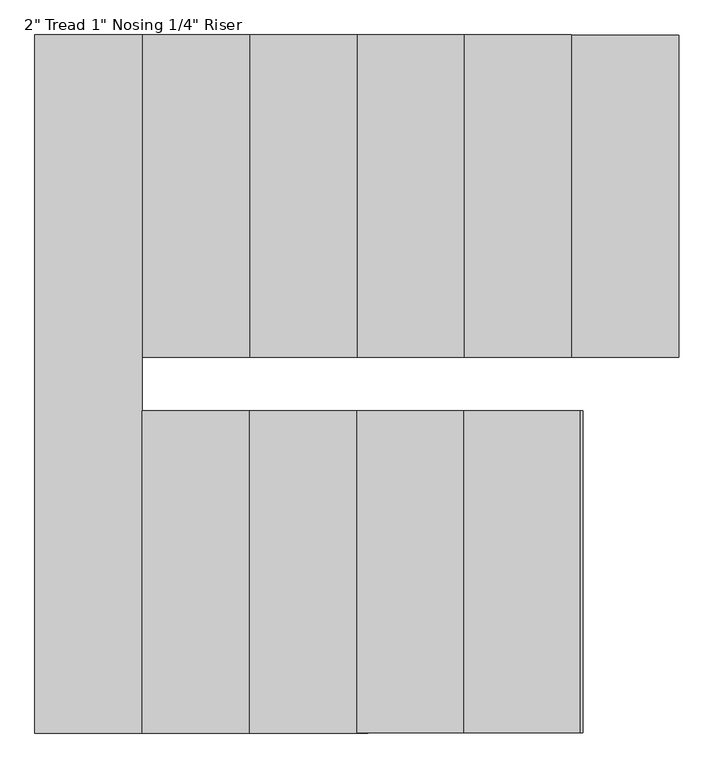
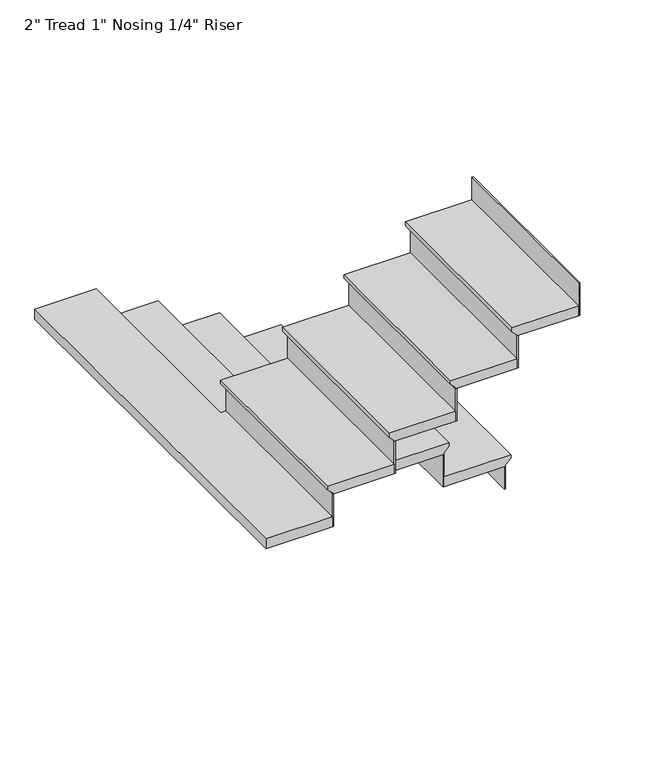
"""IFC4 building model written with IfcOpenShell, lengths in millimetres: stair flight geometry."""

from ifc_helpers import new_model, si_unit, origin, place, context, project, spatial, faceted_brep, source, transform, mapped, element, save


def stair_flight_2df44192(model_context):
    return source(origin(), model_context, "Body", "Brep", [
        faceted_brep([(3327.4, 3340.1, 6246.2833333), (3327.4, 3340.1, 6265.3333333), (3327.4, 2425.7, 6265.3333333), (3327.4, 2425.7, 6246.2833333), (3302.0, 3340.1, 6220.8833333), (3302.0, 2425.7, 6220.8833333), (2997.2, 3340.1, 6265.3333333), (2997.2, 2425.7, 6265.3333333), (3302.0, 2425.7, 6214.5333333), (2997.2, 2425.7, 6214.5333333), (2997.2, 3340.1, 6214.5333333), (3302.0, 3340.1, 6214.5333333)], [[[0, 1, 2, 3]], [[4, 0, 3, 5]], [[2, 1, 6, 7]], [[8, 9, 10, 11]], [[2, 7, 9, 8, 5, 3]], [[8, 11, 4, 5]], [[6, 1, 0, 4, 11, 10]], [[7, 6, 10, 9]]]),
        faceted_brep([(3302.0, 3340.1, 6214.5333333), (3302.0, 3340.1, 6096.0), (3295.65, 3340.1, 6096.0), (3295.65, 3340.1, 6214.5333333), (3302.0, 2425.7, 6214.5333333), (3295.65, 2425.7, 6214.5333333), (3295.65, 2425.7, 6096.0), (3302.0, 2425.7, 6096.0)], [[[0, 1, 2, 3]], [[4, 5, 6, 7]], [[1, 0, 4, 7]], [[2, 1, 7, 6]], [[3, 2, 6, 5]], [[0, 3, 5, 4]]]),
        faceted_brep([(2997.2, 3340.1, 6383.8666667), (2997.2, 3340.1, 6214.5333333), (2990.85, 3340.1, 6214.5333333), (2990.85, 3340.1, 6383.8666667), (2997.2, 2425.7, 6383.8666667), (2990.85, 2425.7, 6383.8666667), (2990.85, 2425.7, 6214.5333333), (2997.2, 2425.7, 6214.5333333)], [[[0, 1, 2, 3]], [[4, 5, 6, 7]], [[1, 0, 4, 7]], [[2, 1, 7, 6]], [[3, 2, 6, 5]], [[0, 3, 5, 4]]]),
        faceted_brep([(3022.6, 2425.7, 6434.6666667), (3022.6, 3340.1, 6434.6666667), (2692.4, 3340.1, 6434.6666667), (2692.4, 2425.7, 6434.6666667), (2997.2, 2425.7, 6383.8666667), (2692.4, 2425.7, 6383.8666667), (2692.4, 3340.1, 6383.8666667), (2997.2, 3340.1, 6383.8666667), (2997.2, 2425.7, 6390.2166667), (3022.6, 2425.7, 6415.6166667), (2997.2, 3340.1, 6390.2166667), (3022.6, 3340.1, 6415.6166667)], [[[0, 1, 2, 3]], [[4, 5, 6, 7]], [[0, 3, 5, 4, 8, 9]], [[4, 7, 10, 8]], [[2, 1, 11, 10, 7, 6]], [[3, 2, 6, 5]], [[11, 1, 0, 9]], [[10, 11, 9, 8]]]),
        faceted_brep([(2692.4, 3340.1, 6553.2), (2692.4, 3340.1, 6383.8666667), (2686.05, 3340.1, 6383.8666667), (2686.05, 3340.1, 6553.2), (2692.4, 2425.7, 6553.2), (2686.05, 2425.7, 6553.2), (2686.05, 2425.7, 6383.8666667), (2692.4, 2425.7, 6383.8666667)], [[[0, 1, 2, 3]], [[4, 5, 6, 7]], [[1, 0, 4, 7]], [[2, 1, 7, 6]], [[3, 2, 6, 5]], [[0, 3, 5, 4]]]),
        faceted_brep([(2717.8, 2425.7, 6604.0), (2717.8, 3340.1, 6604.0), (2387.6, 3340.1, 6604.0), (2387.6, 2425.7, 6604.0), (2692.4, 2425.7, 6553.2), (2387.6, 2425.7, 6553.2), (2387.6, 3340.1, 6553.2), (2692.4, 3340.1, 6553.2), (2692.4, 2425.7, 6559.55), (2717.8, 2425.7, 6584.95), (2692.4, 3340.1, 6559.55), (2717.8, 3340.1, 6584.95)], [[[0, 1, 2, 3]], [[4, 5, 6, 7]], [[0, 3, 5, 4, 8, 9]], [[4, 7, 10, 8]], [[2, 1, 11, 10, 7, 6]], [[3, 2, 6, 5]], [[11, 1, 0, 9]], [[10, 11, 9, 8]]]),
        faceted_brep([(2387.6, 3340.1, 6722.5333333), (2387.6, 3340.1, 6553.2), (2381.25, 3340.1, 6553.2), (2381.25, 3340.1, 6722.5333333), (2387.6, 2425.7, 6722.5333333), (2381.25, 2425.7, 6722.5333333), (2381.25, 2425.7, 6553.2), (2387.6, 2425.7, 6553.2)], [[[0, 1, 2, 3]], [[4, 5, 6, 7]], [[1, 0, 4, 7]], [[2, 1, 7, 6]], [[3, 2, 6, 5]], [[0, 3, 5, 4]]]),
        faceted_brep([(2413.0, 2425.7, 6773.3333333), (2413.0, 3340.1, 6773.3333333), (2082.8, 3340.1, 6773.3333333), (2082.8, 2425.7, 6773.3333333), (2387.6, 2425.7, 6722.5333333), (2082.8, 2425.7, 6722.5333333), (2082.8, 3340.1, 6722.5333333), (2387.6, 3340.1, 6722.5333333), (2387.6, 2425.7, 6728.8833333), (2413.0, 2425.7, 6754.2833333), (2387.6, 3340.1, 6728.8833333), (2413.0, 3340.1, 6754.2833333)], [[[0, 1, 2, 3]], [[4, 5, 6, 7]], [[0, 3, 5, 4, 8, 9]], [[4, 7, 10, 8]], [[2, 1, 11, 10, 7, 6]], [[3, 2, 6, 5]], [[11, 1, 0, 9]], [[10, 11, 9, 8]]]),
        faceted_brep([(2082.8, 3340.1, 6891.8666667), (2082.8, 3340.1, 6722.5333333), (2076.45, 3340.1, 6722.5333333), (2076.45, 3340.1, 6891.8666667), (2082.8, 2425.7, 6891.8666667), (2076.45, 2425.7, 6891.8666667), (2076.45, 2425.7, 6722.5333333), (2082.8, 2425.7, 6722.5333333)], [[[0, 1, 2, 3]], [[4, 5, 6, 7]], [[1, 0, 4, 7]], [[2, 1, 7, 6]], [[3, 2, 6, 5]], [[0, 3, 5, 4]]]),
        faceted_brep([(2108.2, 2425.7, 6942.6666667), (2108.2, 3340.1, 6942.6666667), (1778.0, 3340.1, 6942.6666667), (1778.0, 2425.7, 6942.6666667), (2082.8, 2425.7, 6891.8666667), (1778.0, 2425.7, 6891.8666667), (1778.0, 3340.1, 6891.8666667), (2082.8, 3340.1, 6891.8666667), (2082.8, 2425.7, 6898.2166667), (2108.2, 2425.7, 6923.6166667), (2082.8, 3340.1, 6898.2166667), (2108.2, 3340.1, 6923.6166667)], [[[0, 1, 2, 3]], [[4, 5, 6, 7]], [[0, 3, 5, 4, 8, 9]], [[4, 7, 10, 8]], [[2, 1, 11, 10, 7, 6]], [[3, 2, 6, 5]], [[11, 1, 0, 9]], [[10, 11, 9, 8]]]),
        faceted_brep([(1778.0, 3340.1, 7061.2), (1778.0, 3340.1, 6891.8666667), (1771.65, 3340.1, 6891.8666667), (1771.65, 3340.1, 7061.2), (1778.0, 2425.7, 7061.2), (1771.65, 2425.7, 7061.2), (1771.65, 2425.7, 6891.8666667), (1778.0, 2425.7, 6891.8666667)], [[[0, 1, 2, 3]], [[4, 5, 6, 7]], [[1, 0, 4, 7]], [[2, 1, 7, 6]], [[3, 2, 6, 5]], [[0, 3, 5, 4]]]),
        faceted_brep([(1828.8, 2273.3, 7112.0), (1803.4, 2273.3, 7112.0), (1803.4, 3340.1, 7112.0), (1498.6, 3340.1, 7112.0), (1498.6, 1358.9, 7112.0), (1828.8, 1358.9, 7112.0), (1803.4, 2273.3, 7061.2), (1828.8, 2273.3, 7061.2), (1828.8, 1358.9, 7061.2), (1498.6, 1358.9, 7061.2), (1498.6, 3340.1, 7061.2), (1778.0, 3340.1, 7061.2), (1778.0, 2425.7, 7061.2), (1803.4, 2425.7, 7061.2), (1803.4, 2425.7, 7092.95), (1803.4, 3340.1, 7092.95), (1778.0, 2425.7, 7067.55), (1778.0, 3340.1, 7067.55)], [[[0, 1, 2, 3, 4, 5]], [[6, 7, 8, 9, 10, 11, 12, 13]], [[1, 0, 7, 6]], [[2, 1, 6, 13, 14, 15]], [[13, 12, 16, 14]], [[12, 11, 17, 16]], [[3, 2, 15, 17, 11, 10]], [[4, 3, 10, 9]], [[5, 4, 9, 8]], [[0, 5, 8, 7]], [[17, 15, 14, 16]]]),
        faceted_brep([(1828.8, 1358.9, 7230.5333333), (1828.8, 1358.9, 7061.2), (1835.15, 1358.9, 7061.2), (1835.15, 1358.9, 7230.5333333), (1828.8, 2273.3, 7230.5333333), (1835.15, 2273.3, 7230.5333333), (1835.15, 2273.3, 7061.2), (1828.8, 2273.3, 7061.2)], [[[0, 1, 2, 3]], [[4, 5, 6, 7]], [[1, 0, 4, 7]], [[2, 1, 7, 6]], [[3, 2, 6, 5]], [[0, 3, 5, 4]]]),
        faceted_brep([(1803.4, 2273.3, 7281.3333333), (1803.4, 1358.9, 7281.3333333), (2133.6, 1358.9, 7281.3333333), (2133.6, 2273.3, 7281.3333333), (1828.8, 2273.3, 7230.5333333), (2133.6, 2273.3, 7230.5333333), (2133.6, 1358.9, 7230.5333333), (1828.8, 1358.9, 7230.5333333), (1828.8, 2273.3, 7236.8833333), (1803.4, 2273.3, 7262.2833333), (1828.8, 1358.9, 7236.8833333), (1803.4, 1358.9, 7262.2833333)], [[[0, 1, 2, 3]], [[4, 5, 6, 7]], [[0, 3, 5, 4, 8, 9]], [[4, 7, 10, 8]], [[2, 1, 11, 10, 7, 6]], [[3, 2, 6, 5]], [[11, 1, 0, 9]], [[10, 11, 9, 8]]]),
        faceted_brep([(2133.6, 1358.9, 7399.8666667), (2133.6, 1358.9, 7230.5333333), (2139.95, 1358.9, 7230.5333333), (2139.95, 1358.9, 7399.8666667), (2133.6, 2273.3, 7399.8666667), (2139.95, 2273.3, 7399.8666667), (2139.95, 2273.3, 7230.5333333), (2133.6, 2273.3, 7230.5333333)], [[[0, 1, 2, 3]], [[4, 5, 6, 7]], [[1, 0, 4, 7]], [[2, 1, 7, 6]], [[3, 2, 6, 5]], [[0, 3, 5, 4]]]),
        faceted_brep([(2108.2, 2273.3, 7450.6666667), (2108.2, 1358.9, 7450.6666667), (2438.4, 1358.9, 7450.6666667), (2438.4, 2273.3, 7450.6666667), (2133.6, 2273.3, 7399.8666667), (2438.4, 2273.3, 7399.8666667), (2438.4, 1358.9, 7399.8666667), (2133.6, 1358.9, 7399.8666667), (2133.6, 2273.3, 7406.2166667), (2108.2, 2273.3, 7431.6166667), (2133.6, 1358.9, 7406.2166667), (2108.2, 1358.9, 7431.6166667)], [[[0, 1, 2, 3]], [[4, 5, 6, 7]], [[0, 3, 5, 4, 8, 9]], [[4, 7, 10, 8]], [[2, 1, 11, 10, 7, 6]], [[3, 2, 6, 5]], [[11, 1, 0, 9]], [[10, 11, 9, 8]]]),
        faceted_brep([(2438.4, 1358.9, 7569.2), (2438.4, 1358.9, 7399.8666667), (2444.75, 1358.9, 7399.8666667), (2444.75, 1358.9, 7569.2), (2438.4, 2273.3, 7569.2), (2444.75, 2273.3, 7569.2), (2444.75, 2273.3, 7399.8666667), (2438.4, 2273.3, 7399.8666667)], [[[0, 1, 2, 3]], [[4, 5, 6, 7]], [[1, 0, 4, 7]], [[2, 1, 7, 6]], [[3, 2, 6, 5]], [[0, 3, 5, 4]]]),
        faceted_brep([(2413.0, 2273.3, 7620.0), (2413.0, 1358.9, 7620.0), (2743.2, 1358.9, 7620.0), (2743.2, 2273.3, 7620.0), (2438.4, 2273.3, 7569.2), (2743.2, 2273.3, 7569.2), (2743.2, 1358.9, 7569.2), (2438.4, 1358.9, 7569.2), (2438.4, 2273.3, 7575.55), (2413.0, 2273.3, 7600.95), (2438.4, 1358.9, 7575.55), (2413.0, 1358.9, 7600.95)], [[[0, 1, 2, 3]], [[4, 5, 6, 7]], [[0, 3, 5, 4, 8, 9]], [[4, 7, 10, 8]], [[2, 1, 11, 10, 7, 6]], [[3, 2, 6, 5]], [[11, 1, 0, 9]], [[10, 11, 9, 8]]]),
        faceted_brep([(2743.2, 1358.9, 7738.5333333), (2743.2, 1358.9, 7569.2), (2749.55, 1358.9, 7569.2), (2749.55, 1358.9, 7738.5333333), (2743.2, 2273.3, 7738.5333333), (2749.55, 2273.3, 7738.5333333), (2749.55, 2273.3, 7569.2), (2743.2, 2273.3, 7569.2)], [[[0, 1, 2, 3]], [[4, 5, 6, 7]], [[1, 0, 4, 7]], [[2, 1, 7, 6]], [[3, 2, 6, 5]], [[0, 3, 5, 4]]]),
        faceted_brep([(3048.0, 1358.9, 7907.8666667), (3048.0, 1358.9, 7738.5333333), (3054.35, 1358.9, 7738.5333333), (3054.35, 1358.9, 7907.8666667), (3048.0, 2273.3, 7907.8666667), (3054.35, 2273.3, 7907.8666667), (3054.35, 2273.3, 7738.5333333), (3048.0, 2273.3, 7738.5333333)], [[[0, 1, 2, 3]], [[4, 5, 6, 7]], [[1, 0, 4, 7]], [[2, 1, 7, 6]], [[3, 2, 6, 5]], [[0, 3, 5, 4]]]),
        faceted_brep([(2717.8, 2273.3, 7789.3333333), (2717.8, 1358.9, 7789.3333333), (3048.0, 1358.9, 7789.3333333), (3048.0, 2273.3, 7789.3333333), (2743.2, 2273.3, 7738.5333333), (3048.0, 2273.3, 7738.5333333), (3048.0, 1358.9, 7738.5333333), (2743.2, 1358.9, 7738.5333333), (2743.2, 2273.3, 7744.8833333), (2717.8, 2273.3, 7770.2833333), (2743.2, 1358.9, 7744.8833333), (2717.8, 1358.9, 7770.2833333)], [[[0, 1, 2, 3]], [[4, 5, 6, 7]], [[0, 3, 5, 4, 8, 9]], [[4, 7, 10, 8]], [[2, 1, 11, 10, 7, 6]], [[3, 2, 6, 5]], [[11, 1, 0, 9]], [[10, 11, 9, 8]]]),
    ])


if __name__ == "__main__":
    model = new_model("IFC4")
    model_context = context("Model", 3, world=origin())
    ifc_project = project(units=[si_unit("LENGTHUNIT", "METRE", prefix="MILLI")], contexts=[model_context])
    site = spatial("IfcSite", under=ifc_project)
    building = spatial("IfcBuilding", under=site)
    placement = place(None, origin())
    stair_flight_shape = stair_flight_2df44192(model_context)
    element("IfcStairFlight", 1, ObjectType="2\" Tread 1\" Nosing 1/4\" Riser", at=placement, inside=building, context=model_context, shape_type="MappedRepresentation", body=[
        mapped(stair_flight_shape, transform((0.0, 0.0, 0.0), x_axis=(1.0, 0.0, 0.0), y_axis=(0.0, 1.0, 0.0), z_axis=(0.0, 0.0, 1.0))),
    ])
    save(model, "model.ifc")
